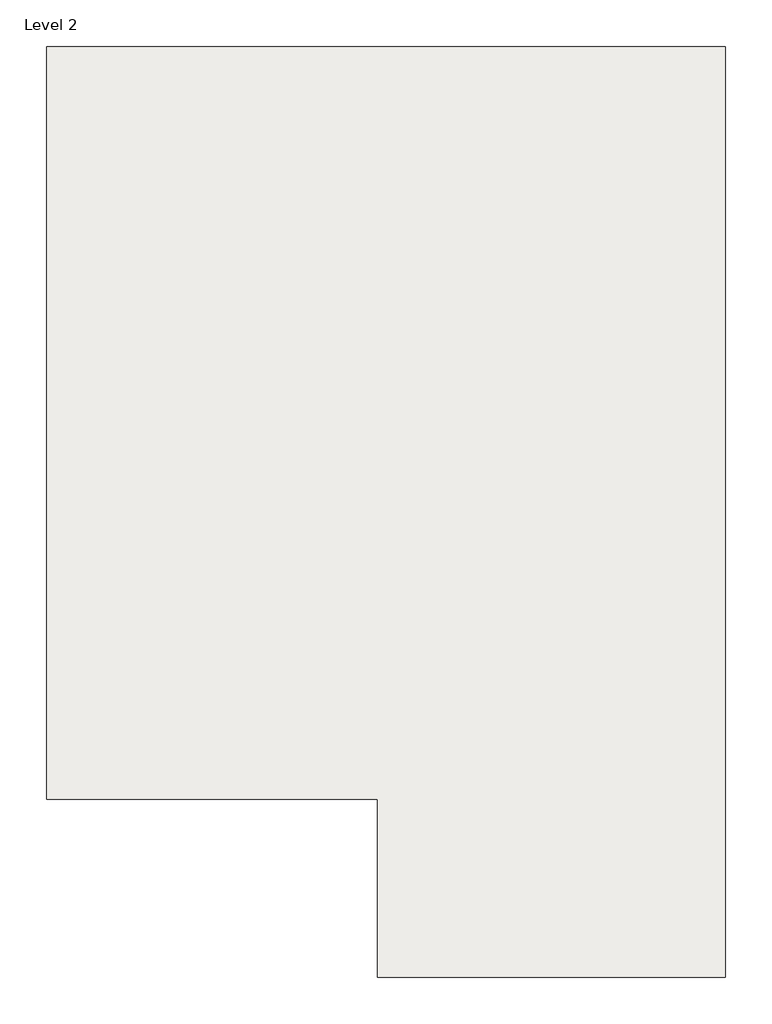
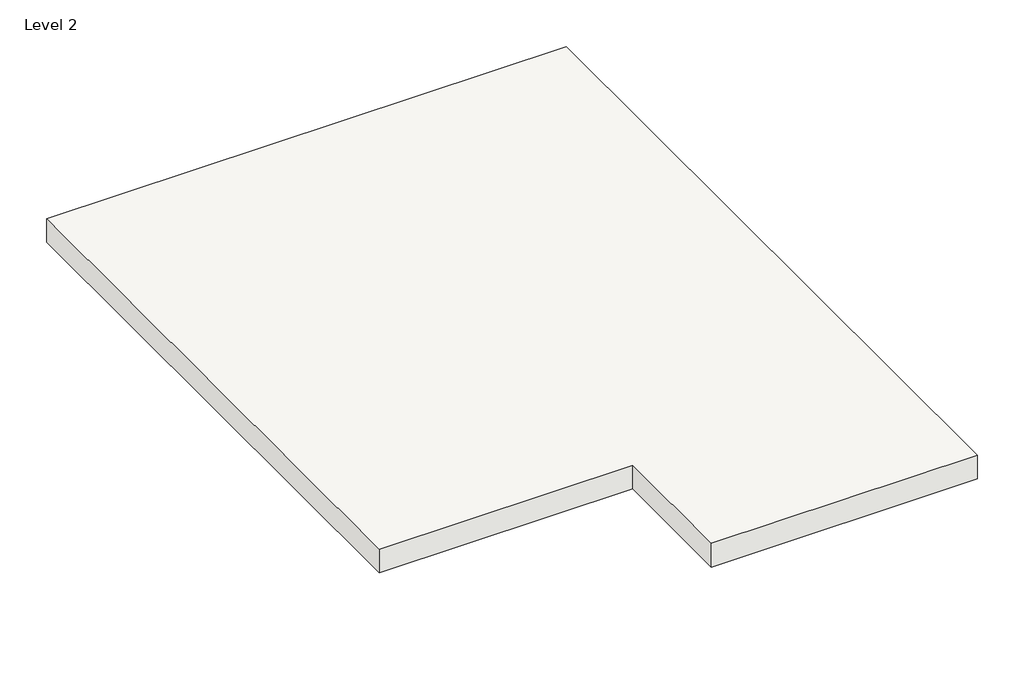
# One storey: 1 roof.
"""IFC4 building model written with IfcOpenShell, lengths in millimetres."""

from ifc_helpers import new_model, si_unit, frame, origin, place, context, project, spatial, polyline, outline, extrude, element, save

model = new_model("IFC4")

# Units and contexts
model_context = context("Model", 3, world=origin())
ifc_project = project(units=[si_unit("LENGTHUNIT", "METRE", prefix="MILLI")], contexts=[model_context])

# Site, building, storey
site = spatial("IfcSite", under=ifc_project)
building = spatial("IfcBuilding", under=site)
storey = spatial("IfcBuildingStorey", under=building, Name="Level 2", Elevation=3048.0)

# Roof
placement = place(None, origin())
element("IfcRoof", 1, ObjectType="Generic - 12\"", at=placement, inside=storey, context=model_context, shape_type="SweptSolid", body=[
    extrude(outline(polyline([(-13440.8586966, 14144.8085318), (-7141.6586966, 14144.8085318), (-7141.6586966, 5508.8085318), (-10367.4586966, 5508.8085318), (-10367.4586966, 7159.8085318), (-13440.8586966, 7159.8085318), (-13440.8586966, 14144.8085318)])), frame((0.0, 0.0, 3048.0), z_axis=(0.0, 0.0, 1.0), x_axis=(1.0, 0.0, 0.0)), (0.0, 0.0, 1.0), 304.8),
])

save(model, "model.ifc")

# Revit data of these elements
# Type "Generic - 12\""
#   Assembly Code = "B1020"
#   Layers, outside or top first: 1' - 0" "Brick, Soldier Course" (function 1)
# Element 1 (IfcRoof, "Generic - 12\"")
#   built-in parameter 1001705 = 11 (stored number, unit not read)
#   built-in parameter 1001710 = 33615
#   Phase Created = New Construction
#   Materials on its faces: "Brick, Soldier Course"
# Materials
#   "Brick, Soldier Course": class "Masonry", colour RGB 170 98 104, transparency 0, Description = "Common brick soldier coursed", Cost = 0
